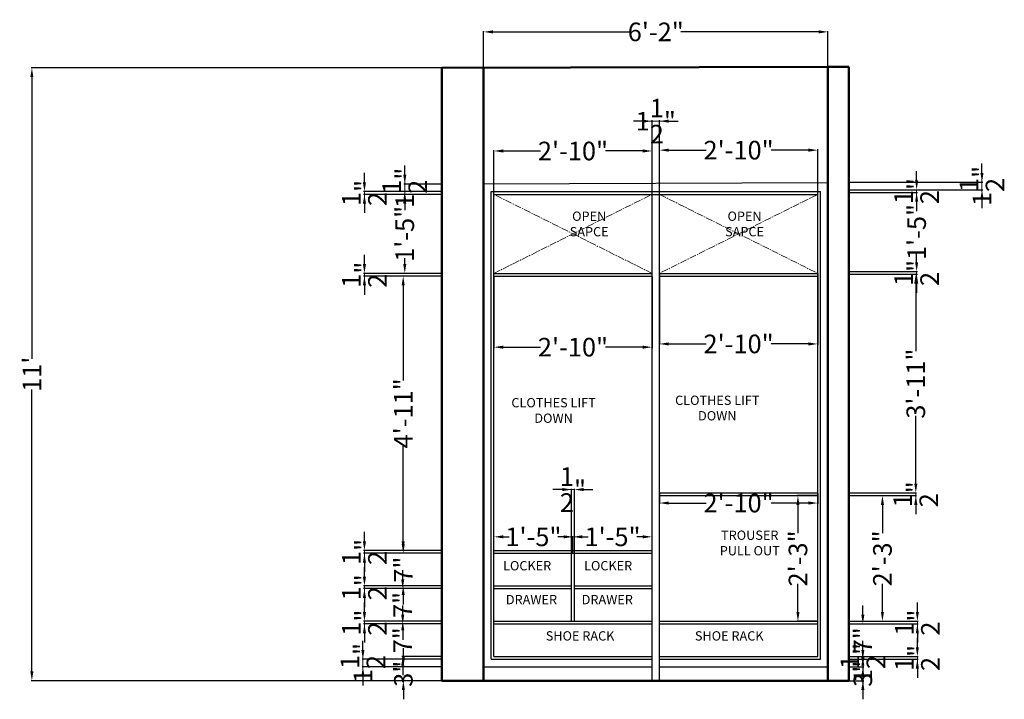
# Model space of a CAD drawing. Units: inches. Extents: x -26 to 186, y 15 to 278.
# Tile 1 of 2: x -26 to 186, y 15 to 161. Entities that reach past the tile are written whole.
import ezdxf

# ---------------------------------------------------------------- set-up
doc = ezdxf.new("R2010")
doc.units = ezdxf.units.IN
doc.header["$LTSCALE"] = 2
doc.header["$MEASUREMENT"] = 0
doc.linetypes.add('CENTER2', pattern=[1.125, 0.75, -0.125, 0.125, -0.125])
for name, color, linetype, lineweight in [('A-ANNO-DIMS', 2, 'Continuous', 18), ('A-ANNO-SYMB', 8, 'CENTER2', 13), ('A-ANNO-TEXT', 7, 'Continuous', 18), ('A-FURN', 3, 'Continuous', 25), ('A-WALL', 7, 'Continuous', 50)]:
    doc.layers.add(name, color=color, linetype=linetype, lineweight=lineweight)
doc.styles.get("Standard").update_dxf_attribs({"font": 'arial.ttf'})
doc.dimstyles.get("Standard").update_dxf_attribs({"dimtxt": 4, "dimasz": 2, "dimexe": 0.18, "dimexo": 0.0625, "dimgap": 0.09, "dimtad": 0, "dimdec": 1, "dimzin": 0, "dimdsep": 46, "dimlunit": 4, "dimtxsty": 'Standard', "dimcen": 0.09, "dimadec": 0, "dimazin": 0, "dimtfac": 1, "dimtdec": 1, "dimtix": 1, "dimtofl": 0, "dimtmove": 1, "dimatfit": 2, "dimfxl": 1, "dimtolj": 1, "dimtzin": 0, "dimarcsym": 0})

# ---------------------------------------------------------------- blocks, each defined once
blk = doc.blocks.new('*D6')
at = {"layer": 'A-ANNO-DIMS', "color": 0, "lineweight": -2, "transparency": 16777216}
for p, q in [((64.89, 150.53), (-23.34, 150.53)), ((-23.16, 148.53), (-23.16, 87.92)), ((-23.16, 20.73), (-23.16, 81.33)), ((64.89, 18.73), (-23.34, 18.73))]:
    blk.add_line(p, q, dxfattribs=at)
at = {"layer": 'A-ANNO-DIMS', "color": 0, "transparency": 16777216}
for points in [[(-23.49, 148.53), (-22.83, 148.53), (-23.16, 150.53)], [(-23.49, 20.73), (-22.83, 20.73), (-23.16, 18.73)]]:
    blk.add_solid(points, dxfattribs=at)
at = {"layer": 'Defpoints', "color": 0, "transparency": 16777216}
for p in [(64.95, 150.53), (-23.16, 18.73), (64.95, 18.73)]:
    blk.add_point(p, dxfattribs=at)
at = {"layer": 'A-ANNO-DIMS', "color": 0, "transparency": 16777216, "insert": (-23.16, 84.63), "char_height": 4, "attachment_point": 5, "rotation": 90}
blk.add_mtext("\\A1;11'", dxfattribs=at)
blk = doc.blocks.new('*D7')
at = {"layer": 'A-ANNO-DIMS', "color": 0, "lineweight": -2, "transparency": 16777216}
for p, q in [((155.46, 23.73), (155.46, 25.73)), ((152.51, 21.73), (155.64, 21.73)), ((152.51, 18.73), (155.64, 18.73)), ((155.46, 16.73), (155.46, 14.73))]:
    blk.add_line(p, q, dxfattribs=at)
at = {"layer": 'A-ANNO-DIMS', "color": 0, "transparency": 16777216}
for points in [[(155.13, 23.73), (155.79, 23.73), (155.46, 21.73)], [(155.13, 16.73), (155.79, 16.73), (155.46, 18.73)]]:
    blk.add_solid(points, dxfattribs=at)
at = {"layer": 'Defpoints', "color": 0, "transparency": 16777216}
for p in [(152.45, 21.73), (152.45, 18.73), (155.46, 18.73)]:
    blk.add_point(p, dxfattribs=at)
at = {"layer": 'A-ANNO-DIMS', "color": 0, "transparency": 16777216, "insert": (155.46, 20.23), "char_height": 4, "attachment_point": 5, "rotation": 90}
blk.add_mtext('\\A1;3"', dxfattribs=at)
blk = doc.blocks.new('*D8')
at = {"layer": 'A-ANNO-DIMS', "color": 0, "lineweight": -2, "transparency": 16777216}
for p, q in [((155.46, 25.33), (155.46, 27.33)), ((152.51, 23.33), (155.64, 23.33)), ((152.51, 21.73), (155.64, 21.73)), ((155.46, 19.73), (155.46, 17.73))]:
    blk.add_line(p, q, dxfattribs=at)
at = {"layer": 'A-ANNO-DIMS', "color": 0, "transparency": 16777216}
for points in [[(155.13, 25.33), (155.79, 25.33), (155.46, 23.33)], [(155.13, 19.73), (155.79, 19.73), (155.46, 21.73)]]:
    blk.add_solid(points, dxfattribs=at)
at = {"layer": 'Defpoints', "color": 0, "transparency": 16777216}
for p in [(152.45, 23.33), (155.46, 23.33), (152.45, 21.73)]:
    blk.add_point(p, dxfattribs=at)
at = {"layer": 'A-ANNO-DIMS', "color": 0, "transparency": 16777216, "insert": (155.46, 22.53), "char_height": 4, "attachment_point": 5, "rotation": 90}
blk.add_mtext('\\A1;1{\\H1x;\\S1/2;}"', dxfattribs=at)
blk = doc.blocks.new('*D9')
at = {"layer": 'A-ANNO-DIMS', "color": 0, "lineweight": -2, "transparency": 16777216}
for p, q in [((167.18, 25.93), (167.18, 27.93)), ((152.51, 23.93), (167.36, 23.93)), ((152.51, 23.33), (167.36, 23.33)), ((167.18, 21.33), (167.18, 19.33))]:
    blk.add_line(p, q, dxfattribs=at)
at = {"layer": 'A-ANNO-DIMS', "color": 0, "transparency": 16777216}
for points in [[(166.84, 25.93), (167.51, 25.93), (167.18, 23.93)], [(166.84, 21.33), (167.51, 21.33), (167.18, 23.33)]]:
    blk.add_solid(points, dxfattribs=at)
at = {"layer": 'Defpoints', "color": 0, "transparency": 16777216}
for p in [(152.45, 23.93), (152.45, 23.33), (167.18, 23.93)]:
    blk.add_point(p, dxfattribs=at)
at = {"layer": 'A-ANNO-DIMS', "color": 0, "transparency": 16777216, "insert": (167.18, 23.63), "char_height": 4, "attachment_point": 5, "rotation": 90}
blk.add_mtext('\\A1;{\\H1x;\\S1/2;}"', dxfattribs=at)
blk = doc.blocks.new('*D10')
at = {"layer": 'A-ANNO-DIMS', "color": 0, "lineweight": -2, "transparency": 16777216}
for p, q in [((155.46, 32.93), (155.46, 34.93)), ((152.51, 30.93), (155.64, 30.93)), ((152.51, 23.93), (155.64, 23.93)), ((155.46, 21.93), (155.46, 19.93))]:
    blk.add_line(p, q, dxfattribs=at)
at = {"layer": 'A-ANNO-DIMS', "color": 0, "transparency": 16777216}
for points in [[(155.13, 32.93), (155.79, 32.93), (155.46, 30.93)], [(155.13, 21.93), (155.79, 21.93), (155.46, 23.93)]]:
    blk.add_solid(points, dxfattribs=at)
at = {"layer": 'Defpoints', "color": 0, "transparency": 16777216}
for p in [(152.45, 30.93), (155.46, 30.93), (152.45, 23.93)]:
    blk.add_point(p, dxfattribs=at)
at = {"layer": 'A-ANNO-DIMS', "color": 0, "transparency": 16777216, "insert": (155.46, 27.43), "char_height": 4, "attachment_point": 5, "rotation": 90}
blk.add_mtext('\\A1;7"', dxfattribs=at)
blk = doc.blocks.new('*D11')
at = {"layer": 'A-ANNO-DIMS', "color": 0, "lineweight": -2, "transparency": 16777216}
for p, q in [((167.18, 33.53), (167.18, 35.53)), ((152.51, 31.53), (167.36, 31.53)), ((152.51, 30.93), (167.36, 30.93)), ((167.18, 28.93), (167.18, 26.93))]:
    blk.add_line(p, q, dxfattribs=at)
at = {"layer": 'A-ANNO-DIMS', "color": 0, "transparency": 16777216}
for points in [[(166.84, 33.53), (167.51, 33.53), (167.18, 31.53)], [(166.84, 28.93), (167.51, 28.93), (167.18, 30.93)]]:
    blk.add_solid(points, dxfattribs=at)
at = {"layer": 'Defpoints', "color": 0, "transparency": 16777216}
for p in [(152.45, 31.53), (152.45, 30.93), (167.18, 31.53)]:
    blk.add_point(p, dxfattribs=at)
at = {"layer": 'A-ANNO-DIMS', "color": 0, "transparency": 16777216, "insert": (167.18, 31.23), "char_height": 4, "attachment_point": 5, "rotation": 90}
blk.add_mtext('\\A1;{\\H1x;\\S1/2;}"', dxfattribs=at)
blk = doc.blocks.new('*D12')
at = {"layer": 'A-ANNO-DIMS', "color": 0, "lineweight": -2, "transparency": 16777216}
for p, q in [((152.51, 58.53), (159.85, 58.53)), ((159.67, 56.53), (159.67, 50.47)), ((159.67, 33.53), (159.67, 39.59)), ((152.51, 31.53), (159.85, 31.53))]:
    blk.add_line(p, q, dxfattribs=at)
at = {"layer": 'A-ANNO-DIMS', "color": 0, "transparency": 16777216}
for points in [[(159.34, 56.53), (160, 56.53), (159.67, 58.53)], [(159.34, 33.53), (160, 33.53), (159.67, 31.53)]]:
    blk.add_solid(points, dxfattribs=at)
at = {"layer": 'Defpoints', "color": 0, "transparency": 16777216}
for p in [(152.45, 58.53), (159.67, 58.53), (152.45, 31.53)]:
    blk.add_point(p, dxfattribs=at)
at = {"layer": 'A-ANNO-DIMS', "color": 0, "transparency": 16777216, "insert": (159.67, 45.03), "char_height": 4, "attachment_point": 5, "rotation": 90}
blk.add_mtext('\\A1;2\'-3"', dxfattribs=at)
blk = doc.blocks.new('*D13')
at = {"layer": 'A-ANNO-DIMS', "color": 0, "lineweight": -2, "transparency": 16777216}
for p, q in [((166.84, 61.13), (166.84, 63.13)), ((152.51, 59.13), (167.02, 59.13)), ((152.51, 58.53), (167.02, 58.53)), ((166.84, 56.53), (166.84, 54.53))]:
    blk.add_line(p, q, dxfattribs=at)
at = {"layer": 'A-ANNO-DIMS', "color": 0, "transparency": 16777216}
for points in [[(166.51, 61.13), (167.18, 61.13), (166.84, 59.13)], [(166.51, 56.53), (167.18, 56.53), (166.84, 58.53)]]:
    blk.add_solid(points, dxfattribs=at)
at = {"layer": 'Defpoints', "color": 0, "transparency": 16777216}
for p in [(152.45, 59.13), (152.45, 58.53), (166.84, 59.13)]:
    blk.add_point(p, dxfattribs=at)
at = {"layer": 'A-ANNO-DIMS', "color": 0, "transparency": 16777216, "insert": (166.84, 58.83), "char_height": 4, "attachment_point": 5, "rotation": 90}
blk.add_mtext('\\A1;{\\H1x;\\S1/2;}"', dxfattribs=at)
blk = doc.blocks.new('*D14')
at = {"layer": 'A-ANNO-DIMS', "color": 0, "lineweight": -2, "transparency": 16777216}
for p, q in [((152.51, 106.13), (167.02, 106.13)), ((166.84, 104.13), (166.84, 89.59)), ((166.84, 61.13), (166.84, 75.67)), ((152.51, 59.13), (167.02, 59.13))]:
    blk.add_line(p, q, dxfattribs=at)
at = {"layer": 'A-ANNO-DIMS', "color": 0, "transparency": 16777216}
for points in [[(166.51, 104.13), (167.18, 104.13), (166.84, 106.13)], [(166.51, 61.13), (167.18, 61.13), (166.84, 59.13)]]:
    blk.add_solid(points, dxfattribs=at)
at = {"layer": 'Defpoints', "color": 0, "transparency": 16777216}
for p in [(152.45, 106.13), (166.84, 106.13), (152.45, 59.13)]:
    blk.add_point(p, dxfattribs=at)
at = {"layer": 'A-ANNO-DIMS', "color": 0, "transparency": 16777216, "insert": (166.84, 82.63), "char_height": 4, "attachment_point": 5, "rotation": 90}
blk.add_mtext('\\A1;3\'-11"', dxfattribs=at)
blk = doc.blocks.new('*D15')
at = {"layer": 'A-ANNO-DIMS', "color": 0, "lineweight": -2, "transparency": 16777216}
for p, q in [((167.02, 108.73), (167.02, 110.73)), ((152.51, 106.73), (167.2, 106.73)), ((152.51, 106.13), (167.2, 106.13)), ((167.02, 104.13), (167.02, 102.13))]:
    blk.add_line(p, q, dxfattribs=at)
at = {"layer": 'A-ANNO-DIMS', "color": 0, "transparency": 16777216}
for points in [[(166.69, 108.73), (167.36, 108.73), (167.02, 106.73)], [(166.69, 104.13), (167.36, 104.13), (167.02, 106.13)]]:
    blk.add_solid(points, dxfattribs=at)
at = {"layer": 'Defpoints', "color": 0, "transparency": 16777216}
for p in [(152.45, 106.73), (152.45, 106.13), (167.02, 106.73)]:
    blk.add_point(p, dxfattribs=at)
at = {"layer": 'A-ANNO-DIMS', "color": 0, "transparency": 16777216, "insert": (167.02, 106.43), "char_height": 4, "attachment_point": 5, "rotation": 90}
blk.add_mtext('\\A1;{\\H1x;\\S1/2;}"', dxfattribs=at)
blk = doc.blocks.new('*D16')
at = {"layer": 'A-ANNO-DIMS', "color": 0, "lineweight": -2, "transparency": 16777216}
for p, q in [((152.51, 123.73), (167.2, 123.73)), ((167.02, 121.73), (167.02, 120.45)), ((167.02, 108.73), (167.02, 110.01)), ((152.51, 106.73), (167.2, 106.73))]:
    blk.add_line(p, q, dxfattribs=at)
at = {"layer": 'A-ANNO-DIMS', "color": 0, "transparency": 16777216}
for points in [[(166.69, 121.73), (167.36, 121.73), (167.02, 123.73)], [(166.69, 108.73), (167.36, 108.73), (167.02, 106.73)]]:
    blk.add_solid(points, dxfattribs=at)
at = {"layer": 'Defpoints', "color": 0, "transparency": 16777216}
for p in [(152.45, 123.73), (167.02, 123.73), (152.45, 106.73)]:
    blk.add_point(p, dxfattribs=at)
at = {"layer": 'A-ANNO-DIMS', "color": 0, "transparency": 16777216, "insert": (167.02, 115.23), "char_height": 4, "attachment_point": 5, "rotation": 90}
blk.add_mtext('\\A1;1\'-5"', dxfattribs=at)
blk = doc.blocks.new('*D17')
at = {"layer": 'A-ANNO-DIMS', "color": 0, "lineweight": -2, "transparency": 16777216}
for p, q in [((167.02, 126.33), (167.02, 128.33)), ((152.51, 124.33), (167.2, 124.33)), ((152.51, 123.73), (167.2, 123.73)), ((167.02, 121.73), (167.02, 119.73))]:
    blk.add_line(p, q, dxfattribs=at)
at = {"layer": 'A-ANNO-DIMS', "color": 0, "transparency": 16777216}
for points in [[(166.69, 126.33), (167.36, 126.33), (167.02, 124.33)], [(166.69, 121.73), (167.36, 121.73), (167.02, 123.73)]]:
    blk.add_solid(points, dxfattribs=at)
at = {"layer": 'Defpoints', "color": 0, "transparency": 16777216}
for p in [(152.45, 124.33), (152.45, 123.73), (167.02, 124.33)]:
    blk.add_point(p, dxfattribs=at)
at = {"layer": 'A-ANNO-DIMS', "color": 0, "transparency": 16777216, "insert": (167.02, 124.03), "char_height": 4, "attachment_point": 5, "rotation": 90}
blk.add_mtext('\\A1;{\\H1x;\\S1/2;}"', dxfattribs=at)
blk = doc.blocks.new('*D18')
at = {"layer": 'A-ANNO-DIMS', "color": 0, "lineweight": -2, "transparency": 16777216}
for p, q in [((181.07, 127.93), (181.07, 129.93)), ((152.51, 125.93), (181.25, 125.93)), ((152.51, 124.33), (181.25, 124.33)), ((181.07, 122.33), (181.07, 120.33))]:
    blk.add_line(p, q, dxfattribs=at)
at = {"layer": 'A-ANNO-DIMS', "color": 0, "transparency": 16777216}
for points in [[(180.73, 127.93), (181.4, 127.93), (181.07, 125.93)], [(180.73, 122.33), (181.4, 122.33), (181.07, 124.33)]]:
    blk.add_solid(points, dxfattribs=at)
at = {"layer": 'Defpoints', "color": 0, "transparency": 16777216}
for p in [(152.45, 125.93), (181.07, 125.93), (152.45, 124.33)]:
    blk.add_point(p, dxfattribs=at)
at = {"layer": 'A-ANNO-DIMS', "color": 0, "transparency": 16777216, "insert": (181.07, 125.13), "char_height": 4, "attachment_point": 5, "rotation": 90}
blk.add_mtext('\\A1;1{\\H1x;\\S1/2;}"', dxfattribs=at)
blk = doc.blocks.new('*D19')
at = {"layer": 'A-ANNO-DIMS', "color": 0, "lineweight": -2, "transparency": 16777216}
for p, q in [((56.69, 23.73), (56.69, 25.73)), ((64.89, 21.73), (56.51, 21.73)), ((64.89, 18.73), (56.51, 18.73)), ((56.69, 16.73), (56.69, 14.73))]:
    blk.add_line(p, q, dxfattribs=at)
at = {"layer": 'A-ANNO-DIMS', "color": 0, "transparency": 16777216}
for points in [[(56.36, 23.73), (57.02, 23.73), (56.69, 21.73)], [(56.36, 16.73), (57.02, 16.73), (56.69, 18.73)]]:
    blk.add_solid(points, dxfattribs=at)
at = {"layer": 'Defpoints', "color": 0, "transparency": 16777216}
for p in [(56.69, 21.73), (64.95, 21.73), (64.95, 18.73)]:
    blk.add_point(p, dxfattribs=at)
at = {"layer": 'A-ANNO-DIMS', "color": 0, "transparency": 16777216, "insert": (56.69, 20.23), "char_height": 4, "attachment_point": 5, "rotation": 90}
blk.add_mtext('\\A1;3"', dxfattribs=at)
blk = doc.blocks.new('*D20')
at = {"layer": 'A-ANNO-DIMS', "color": 0, "lineweight": -2, "transparency": 16777216}
for p, q in [((47.99, 25.33), (47.99, 27.33)), ((64.89, 23.33), (47.81, 23.33)), ((64.89, 21.73), (47.81, 21.73)), ((47.99, 19.73), (47.99, 17.73))]:
    blk.add_line(p, q, dxfattribs=at)
at = {"layer": 'A-ANNO-DIMS', "color": 0, "transparency": 16777216}
for points in [[(47.66, 25.33), (48.32, 25.33), (47.99, 23.33)], [(47.66, 19.73), (48.32, 19.73), (47.99, 21.73)]]:
    blk.add_solid(points, dxfattribs=at)
at = {"layer": 'Defpoints', "color": 0, "transparency": 16777216}
for p in [(47.99, 23.33), (64.95, 23.33), (64.95, 21.73)]:
    blk.add_point(p, dxfattribs=at)
at = {"layer": 'A-ANNO-DIMS', "color": 0, "transparency": 16777216, "insert": (47.99, 22.53), "char_height": 4, "attachment_point": 5, "rotation": 90}
blk.add_mtext('\\A1;1{\\H1x;\\S1/2;}"', dxfattribs=at)
blk = doc.blocks.new('*D21')
at = {"layer": 'A-ANNO-DIMS', "color": 0, "lineweight": -2, "transparency": 16777216}
for p, q in [((56.56, 32.93), (56.56, 34.93)), ((64.89, 30.93), (56.38, 30.93)), ((64.89, 23.93), (56.38, 23.93)), ((56.56, 21.93), (56.56, 19.93))]:
    blk.add_line(p, q, dxfattribs=at)
at = {"layer": 'A-ANNO-DIMS', "color": 0, "transparency": 16777216}
for points in [[(56.22, 32.93), (56.89, 32.93), (56.56, 30.93)], [(56.22, 21.93), (56.89, 21.93), (56.56, 23.93)]]:
    blk.add_solid(points, dxfattribs=at)
at = {"layer": 'Defpoints', "color": 0, "transparency": 16777216}
for p in [(56.56, 30.93), (64.95, 30.93), (64.95, 23.93)]:
    blk.add_point(p, dxfattribs=at)
at = {"layer": 'A-ANNO-DIMS', "color": 0, "transparency": 16777216, "insert": (56.56, 27.43), "char_height": 4, "attachment_point": 5, "rotation": 90}
blk.add_mtext('\\A1;7"', dxfattribs=at)
blk = doc.blocks.new('*D22')
at = {"layer": 'A-ANNO-DIMS', "color": 0, "lineweight": -2, "transparency": 16777216}
for p, q in [((48.32, 33.53), (48.32, 35.53)), ((64.89, 31.53), (48.14, 31.53)), ((64.89, 30.93), (48.14, 30.93)), ((48.32, 28.93), (48.32, 26.93))]:
    blk.add_line(p, q, dxfattribs=at)
at = {"layer": 'A-ANNO-DIMS', "color": 0, "transparency": 16777216}
for points in [[(47.99, 33.53), (48.66, 33.53), (48.32, 31.53)], [(47.99, 28.93), (48.66, 28.93), (48.32, 30.93)]]:
    blk.add_solid(points, dxfattribs=at)
at = {"layer": 'Defpoints', "color": 0, "transparency": 16777216}
for p in [(48.32, 31.53), (64.95, 31.53), (64.95, 30.93)]:
    blk.add_point(p, dxfattribs=at)
at = {"layer": 'A-ANNO-DIMS', "color": 0, "transparency": 16777216, "insert": (48.32, 31.23), "char_height": 4, "attachment_point": 5, "rotation": 90}
blk.add_mtext('\\A1;{\\H1x;\\S1/2;}"', dxfattribs=at)
blk = doc.blocks.new('*D23')
at = {"layer": 'A-ANNO-DIMS', "color": 0, "lineweight": -2, "transparency": 16777216}
for p, q in [((56.56, 40.53), (56.56, 42.53)), ((64.89, 38.53), (56.38, 38.53)), ((64.89, 31.53), (56.38, 31.53)), ((56.56, 29.53), (56.56, 27.53))]:
    blk.add_line(p, q, dxfattribs=at)
at = {"layer": 'A-ANNO-DIMS', "color": 0, "transparency": 16777216}
for points in [[(56.22, 40.53), (56.89, 40.53), (56.56, 38.53)], [(56.22, 29.53), (56.89, 29.53), (56.56, 31.53)]]:
    blk.add_solid(points, dxfattribs=at)
at = {"layer": 'Defpoints', "color": 0, "transparency": 16777216}
for p in [(56.56, 38.53), (64.95, 38.53), (64.95, 31.53)]:
    blk.add_point(p, dxfattribs=at)
at = {"layer": 'A-ANNO-DIMS', "color": 0, "transparency": 16777216, "insert": (56.56, 35.03), "char_height": 4, "attachment_point": 5, "rotation": 90}
blk.add_mtext('\\A1;7"', dxfattribs=at)
blk = doc.blocks.new('*D24')
at = {"layer": 'A-ANNO-DIMS', "color": 0, "lineweight": -2, "transparency": 16777216}
for p, q in [((48.32, 41.13), (48.32, 43.13)), ((64.89, 39.13), (48.14, 39.13)), ((64.89, 38.53), (48.14, 38.53)), ((48.32, 36.53), (48.32, 34.53))]:
    blk.add_line(p, q, dxfattribs=at)
at = {"layer": 'A-ANNO-DIMS', "color": 0, "transparency": 16777216}
for points in [[(47.99, 41.13), (48.66, 41.13), (48.32, 39.13)], [(47.99, 36.53), (48.66, 36.53), (48.32, 38.53)]]:
    blk.add_solid(points, dxfattribs=at)
at = {"layer": 'Defpoints', "color": 0, "transparency": 16777216}
for p in [(48.32, 39.13), (64.95, 39.13), (64.95, 38.53)]:
    blk.add_point(p, dxfattribs=at)
at = {"layer": 'A-ANNO-DIMS', "color": 0, "transparency": 16777216, "insert": (48.32, 38.83), "char_height": 4, "attachment_point": 5, "rotation": 90}
blk.add_mtext('\\A1;{\\H1x;\\S1/2;}"', dxfattribs=at)
blk = doc.blocks.new('*D25')
at = {"layer": 'A-ANNO-DIMS', "color": 0, "lineweight": -2, "transparency": 16777216}
for p, q in [((56.66, 48.13), (56.66, 50.13)), ((64.89, 46.13), (56.48, 46.13)), ((64.89, 39.13), (56.48, 39.13)), ((56.66, 37.13), (56.66, 35.13))]:
    blk.add_line(p, q, dxfattribs=at)
at = {"layer": 'A-ANNO-DIMS', "color": 0, "transparency": 16777216}
for points in [[(56.32, 48.13), (56.99, 48.13), (56.66, 46.13)], [(56.32, 37.13), (56.99, 37.13), (56.66, 39.13)]]:
    blk.add_solid(points, dxfattribs=at)
at = {"layer": 'Defpoints', "color": 0, "transparency": 16777216}
for p in [(56.66, 46.13), (64.95, 46.13), (64.95, 39.13)]:
    blk.add_point(p, dxfattribs=at)
at = {"layer": 'A-ANNO-DIMS', "color": 0, "transparency": 16777216, "insert": (56.66, 42.63), "char_height": 4, "attachment_point": 5, "rotation": 90}
blk.add_mtext('\\A1;7"', dxfattribs=at)
blk = doc.blocks.new('*D26')
at = {"layer": 'A-ANNO-DIMS', "color": 0, "lineweight": -2, "transparency": 16777216}
for p, q in [((48.32, 48.73), (48.32, 50.73)), ((64.89, 46.73), (48.14, 46.73)), ((64.89, 46.13), (48.14, 46.13)), ((48.32, 44.13), (48.32, 42.13))]:
    blk.add_line(p, q, dxfattribs=at)
at = {"layer": 'A-ANNO-DIMS', "color": 0, "transparency": 16777216}
for points in [[(47.99, 48.73), (48.66, 48.73), (48.32, 46.73)], [(47.99, 44.13), (48.66, 44.13), (48.32, 46.13)]]:
    blk.add_solid(points, dxfattribs=at)
at = {"layer": 'Defpoints', "color": 0, "transparency": 16777216}
for p in [(48.32, 46.73), (64.95, 46.73), (64.95, 46.13)]:
    blk.add_point(p, dxfattribs=at)
at = {"layer": 'A-ANNO-DIMS', "color": 0, "transparency": 16777216, "insert": (48.32, 46.43), "char_height": 4, "attachment_point": 5, "rotation": 90}
blk.add_mtext('\\A1;{\\H1x;\\S1/2;}"', dxfattribs=at)
blk = doc.blocks.new('*D27')
at = {"layer": 'A-ANNO-DIMS', "color": 0, "lineweight": -2, "transparency": 16777216}
for p, q in [((48.32, 108.33), (48.32, 110.33)), ((64.89, 106.33), (48.14, 106.33)), ((64.89, 105.73), (48.14, 105.73)), ((48.32, 103.73), (48.32, 101.73))]:
    blk.add_line(p, q, dxfattribs=at)
at = {"layer": 'A-ANNO-DIMS', "color": 0, "transparency": 16777216}
for points in [[(47.99, 108.33), (48.66, 108.33), (48.32, 106.33)], [(47.99, 103.73), (48.66, 103.73), (48.32, 105.73)]]:
    blk.add_solid(points, dxfattribs=at)
at = {"layer": 'Defpoints', "color": 0, "transparency": 16777216}
for p in [(48.32, 106.33), (64.95, 106.33), (64.95, 105.73)]:
    blk.add_point(p, dxfattribs=at)
at = {"layer": 'A-ANNO-DIMS', "color": 0, "transparency": 16777216, "insert": (48.32, 106.03), "char_height": 4, "attachment_point": 5, "rotation": 90}
blk.add_mtext('\\A1;{\\H1x;\\S1/2;}"', dxfattribs=at)
blk = doc.blocks.new('*D28')
at = {"layer": 'A-ANNO-DIMS', "color": 0, "lineweight": -2, "transparency": 16777216}
for p, q in [((64.89, 105.73), (56.48, 105.73)), ((56.66, 103.73), (56.66, 83.27)), ((56.66, 48.73), (56.66, 69.19)), ((64.89, 46.73), (56.48, 46.73))]:
    blk.add_line(p, q, dxfattribs=at)
at = {"layer": 'A-ANNO-DIMS', "color": 0, "transparency": 16777216}
for points in [[(56.32, 103.73), (56.99, 103.73), (56.66, 105.73)], [(56.32, 48.73), (56.99, 48.73), (56.66, 46.73)]]:
    blk.add_solid(points, dxfattribs=at)
at = {"layer": 'Defpoints', "color": 0, "transparency": 16777216}
for p in [(56.66, 105.73), (64.95, 105.73), (64.95, 46.73)]:
    blk.add_point(p, dxfattribs=at)
at = {"layer": 'A-ANNO-DIMS', "color": 0, "transparency": 16777216, "insert": (56.66, 76.23), "char_height": 4, "attachment_point": 5, "rotation": 90}
blk.add_mtext('\\A1;4\'-11"', dxfattribs=at)
blk = doc.blocks.new('*D29')
at = {"layer": 'A-ANNO-DIMS', "color": 0, "lineweight": -2, "transparency": 16777216}
for p, q in [((64.89, 123.33), (56.81, 123.33)), ((56.99, 121.33), (56.99, 120.05)), ((56.99, 108.33), (56.99, 109.61)), ((64.89, 106.33), (56.81, 106.33))]:
    blk.add_line(p, q, dxfattribs=at)
at = {"layer": 'A-ANNO-DIMS', "color": 0, "transparency": 16777216}
for points in [[(56.66, 121.33), (57.32, 121.33), (56.99, 123.33)], [(56.66, 108.33), (57.32, 108.33), (56.99, 106.33)]]:
    blk.add_solid(points, dxfattribs=at)
at = {"layer": 'Defpoints', "color": 0, "transparency": 16777216}
for p in [(56.99, 123.33), (64.95, 123.33), (64.95, 106.33)]:
    blk.add_point(p, dxfattribs=at)
at = {"layer": 'A-ANNO-DIMS', "color": 0, "transparency": 16777216, "insert": (56.99, 114.83), "char_height": 4, "attachment_point": 5, "rotation": 90}
blk.add_mtext('\\A1;1\'-5"', dxfattribs=at)
blk = doc.blocks.new('*D30')
at = {"layer": 'A-ANNO-DIMS', "color": 0, "lineweight": -2, "transparency": 16777216}
for p, q in [((48.32, 125.93), (48.32, 127.93)), ((64.89, 123.93), (48.14, 123.93)), ((64.89, 123.33), (48.14, 123.33)), ((48.32, 121.33), (48.32, 119.33))]:
    blk.add_line(p, q, dxfattribs=at)
at = {"layer": 'A-ANNO-DIMS', "color": 0, "transparency": 16777216}
for points in [[(47.99, 125.93), (48.66, 125.93), (48.32, 123.93)], [(47.99, 121.33), (48.66, 121.33), (48.32, 123.33)]]:
    blk.add_solid(points, dxfattribs=at)
at = {"layer": 'Defpoints', "color": 0, "transparency": 16777216}
for p in [(48.32, 123.93), (64.95, 123.93), (64.95, 123.33)]:
    blk.add_point(p, dxfattribs=at)
at = {"layer": 'A-ANNO-DIMS', "color": 0, "transparency": 16777216, "insert": (48.32, 123.63), "char_height": 4, "attachment_point": 5, "rotation": 90}
blk.add_mtext('\\A1;{\\H1x;\\S1/2;}"', dxfattribs=at)
blk = doc.blocks.new('*D31')
at = {"layer": 'A-ANNO-DIMS', "color": 0, "lineweight": -2, "transparency": 16777216}
for p, q in [((56.99, 127.53), (56.99, 129.53)), ((64.89, 125.53), (56.81, 125.53)), ((64.89, 123.93), (56.81, 123.93)), ((56.99, 121.93), (56.99, 119.93))]:
    blk.add_line(p, q, dxfattribs=at)
at = {"layer": 'A-ANNO-DIMS', "color": 0, "transparency": 16777216}
for points in [[(56.66, 127.53), (57.32, 127.53), (56.99, 125.53)], [(56.66, 121.93), (57.32, 121.93), (56.99, 123.93)]]:
    blk.add_solid(points, dxfattribs=at)
at = {"layer": 'Defpoints', "color": 0, "transparency": 16777216}
for p in [(56.99, 125.53), (64.95, 125.53), (64.95, 123.93)]:
    blk.add_point(p, dxfattribs=at)
at = {"layer": 'A-ANNO-DIMS', "color": 0, "transparency": 16777216, "insert": (56.99, 124.73), "char_height": 4, "attachment_point": 5, "rotation": 90}
blk.add_mtext('\\A1;1{\\H1x;\\S1/2;}"', dxfattribs=at)
blk = doc.blocks.new('*D32')
at = {"layer": 'A-ANNO-DIMS', "color": 0, "lineweight": -2, "transparency": 16777216}
for p, q in [((76.15, 46.19), (76.15, 49.85)), ((78.15, 49.67), (79.43, 49.67)), ((91.15, 49.67), (89.87, 49.67)), ((93.15, 46.19), (93.15, 49.85))]:
    blk.add_line(p, q, dxfattribs=at)
at = {"layer": 'A-ANNO-DIMS', "color": 0, "transparency": 16777216}
for points in [[(78.15, 50), (78.15, 49.34), (76.15, 49.67)], [(91.15, 50), (91.15, 49.34), (93.15, 49.67)]]:
    blk.add_solid(points, dxfattribs=at)
at = {"layer": 'Defpoints', "color": 0, "transparency": 16777216}
for p in [(93.15, 49.67), (76.15, 46.13), (93.15, 46.13)]:
    blk.add_point(p, dxfattribs=at)
at = {"layer": 'A-ANNO-DIMS', "color": 0, "transparency": 16777216, "insert": (84.65, 49.67), "char_height": 4, "attachment_point": 5}
blk.add_mtext('\\A1;1\'-5"', dxfattribs=at)
blk = doc.blocks.new('*D33')
at = {"layer": 'A-ANNO-DIMS', "color": 0, "lineweight": -2, "transparency": 16777216}
for p, q in [((93.15, 46.19), (93.15, 49.85)), ((95.15, 49.67), (96.43, 49.67)), ((108.15, 49.67), (106.87, 49.67)), ((110.15, 46.19), (110.15, 49.85))]:
    blk.add_line(p, q, dxfattribs=at)
at = {"layer": 'A-ANNO-DIMS', "color": 0, "transparency": 16777216}
for points in [[(95.15, 50), (95.15, 49.34), (93.15, 49.67)], [(108.15, 50), (108.15, 49.34), (110.15, 49.67)]]:
    blk.add_solid(points, dxfattribs=at)
at = {"layer": 'Defpoints', "color": 0, "transparency": 16777216}
for p in [(110.15, 49.67), (93.15, 46.13), (110.15, 46.13)]:
    blk.add_point(p, dxfattribs=at)
at = {"layer": 'A-ANNO-DIMS', "color": 0, "transparency": 16777216, "insert": (101.65, 49.67), "char_height": 4, "attachment_point": 5}
blk.add_mtext('\\A1;1\'-5"', dxfattribs=at)
blk = doc.blocks.new('*D34')
at = {"layer": 'A-ANNO-DIMS', "color": 0, "lineweight": -2, "transparency": 16777216}
for p, q in [((73.95, 150.79), (73.95, 158.45)), ((75.95, 158.27), (105.53, 158.27)), ((145.95, 158.27), (116.37, 158.27)), ((147.95, 150.79), (147.95, 158.45))]:
    blk.add_line(p, q, dxfattribs=at)
at = {"layer": 'A-ANNO-DIMS', "color": 0, "transparency": 16777216}
for points in [[(75.95, 158.6), (75.95, 157.93), (73.95, 158.27)], [(145.95, 158.6), (145.95, 157.93), (147.95, 158.27)]]:
    blk.add_solid(points, dxfattribs=at)
at = {"layer": 'Defpoints', "color": 0, "transparency": 16777216}
for p in [(147.95, 158.27), (73.95, 150.73), (147.95, 150.73)]:
    blk.add_point(p, dxfattribs=at)
at = {"layer": 'A-ANNO-DIMS', "color": 0, "transparency": 16777216, "insert": (110.95, 158.27), "char_height": 4, "attachment_point": 5}
blk.add_mtext('\\A1;6\'-2"', dxfattribs=at)
blk = doc.blocks.new('*D35')
at = {"layer": 'A-ANNO-DIMS', "color": 0, "lineweight": -2, "transparency": 16777216}
for p, q in [((76.15, 123.39), (76.15, 132.83)), ((78.15, 132.65), (86.15, 132.65)), ((108.15, 132.65), (100.14, 132.65)), ((110.15, 123.39), (110.15, 132.83))]:
    blk.add_line(p, q, dxfattribs=at)
at = {"layer": 'A-ANNO-DIMS', "color": 0, "transparency": 16777216}
for points in [[(78.15, 132.99), (78.15, 132.32), (76.15, 132.65)], [(108.15, 132.99), (108.15, 132.32), (110.15, 132.65)]]:
    blk.add_solid(points, dxfattribs=at)
at = {"layer": 'Defpoints', "color": 0, "transparency": 16777216}
for p in [(76.15, 132.65), (76.15, 123.33), (110.15, 123.33)]:
    blk.add_point(p, dxfattribs=at)
at = {"layer": 'A-ANNO-DIMS', "color": 0, "transparency": 16777216, "insert": (93.15, 132.65), "char_height": 4, "attachment_point": 5}
blk.add_mtext('\\A1;2\'-10"', dxfattribs=at)
blk = doc.blocks.new('*D36')
at = {"layer": 'A-ANNO-DIMS', "color": 0, "lineweight": -2, "transparency": 16777216}
for p, q in [((111.75, 123.39), (111.75, 133.01)), ((113.75, 132.83), (121.75, 132.83)), ((143.75, 132.83), (135.74, 132.83)), ((145.75, 123.39), (145.75, 133.01))]:
    blk.add_line(p, q, dxfattribs=at)
at = {"layer": 'A-ANNO-DIMS', "color": 0, "transparency": 16777216}
for points in [[(113.75, 133.17), (113.75, 132.5), (111.75, 132.83)], [(143.75, 133.17), (143.75, 132.5), (145.75, 132.83)]]:
    blk.add_solid(points, dxfattribs=at)
at = {"layer": 'Defpoints', "color": 0, "transparency": 16777216}
for p in [(145.75, 132.83), (111.75, 123.33), (145.75, 123.33)]:
    blk.add_point(p, dxfattribs=at)
at = {"layer": 'A-ANNO-DIMS', "color": 0, "transparency": 16777216, "insert": (128.75, 132.83), "char_height": 4, "attachment_point": 5}
blk.add_mtext('\\A1;2\'-10"', dxfattribs=at)
blk = doc.blocks.new('*D37')
at = {"layer": 'A-ANNO-DIMS', "color": 0, "lineweight": -2, "transparency": 16777216}
for p, q in [((76.15, 105.67), (76.15, 90.28)), ((110.15, 105.67), (110.15, 90.28)), ((78.15, 90.46), (86.15, 90.46)), ((108.15, 90.46), (100.14, 90.46))]:
    blk.add_line(p, q, dxfattribs=at)
at = {"layer": 'A-ANNO-DIMS', "color": 0, "transparency": 16777216}
for points in [[(78.15, 90.79), (78.15, 90.13), (76.15, 90.46)], [(108.15, 90.79), (108.15, 90.13), (110.15, 90.46)]]:
    blk.add_solid(points, dxfattribs=at)
at = {"layer": 'Defpoints', "color": 0, "transparency": 16777216}
for p in [(76.15, 105.73), (110.15, 105.73), (110.15, 90.46)]:
    blk.add_point(p, dxfattribs=at)
at = {"layer": 'A-ANNO-DIMS', "color": 0, "transparency": 16777216, "insert": (93.15, 90.46), "char_height": 4, "attachment_point": 5}
blk.add_mtext('\\A1;2\'-10"', dxfattribs=at)
blk = doc.blocks.new('*D38')
at = {"layer": 'A-ANNO-DIMS', "color": 0, "lineweight": -2, "transparency": 16777216}
for p, q in [((111.75, 106.27), (111.75, 90.98)), ((145.75, 106.27), (145.75, 90.98)), ((113.75, 91.16), (121.75, 91.16)), ((143.75, 91.16), (135.74, 91.16))]:
    blk.add_line(p, q, dxfattribs=at)
at = {"layer": 'A-ANNO-DIMS', "color": 0, "transparency": 16777216}
for points in [[(113.75, 91.49), (113.75, 90.82), (111.75, 91.16)], [(143.75, 91.49), (143.75, 90.82), (145.75, 91.16)]]:
    blk.add_solid(points, dxfattribs=at)
at = {"layer": 'Defpoints', "color": 0, "transparency": 16777216}
for p in [(111.75, 106.33), (145.75, 106.33), (145.75, 91.16)]:
    blk.add_point(p, dxfattribs=at)
at = {"layer": 'A-ANNO-DIMS', "color": 0, "transparency": 16777216, "insert": (128.75, 91.16), "char_height": 4, "attachment_point": 5}
blk.add_mtext('\\A1;2\'-10"', dxfattribs=at)
blk = doc.blocks.new('*D39')
at = {"layer": 'A-ANNO-DIMS', "color": 0, "lineweight": -2, "transparency": 16777216}
for p, q in [((90.85, 59.84), (88.85, 59.84)), ((92.85, 46.19), (92.85, 60.02)), ((93.45, 46.19), (93.45, 60.02)), ((95.45, 59.84), (97.45, 59.84))]:
    blk.add_line(p, q, dxfattribs=at)
at = {"layer": 'A-ANNO-DIMS', "color": 0, "transparency": 16777216}
for points in [[(90.85, 60.18), (90.85, 59.51), (92.85, 59.84)], [(95.45, 60.18), (95.45, 59.51), (93.45, 59.84)]]:
    blk.add_solid(points, dxfattribs=at)
at = {"layer": 'Defpoints', "color": 0, "transparency": 16777216}
for p in [(93.45, 59.84), (92.85, 46.13), (93.45, 46.13)]:
    blk.add_point(p, dxfattribs=at)
at = {"layer": 'A-ANNO-DIMS', "color": 0, "transparency": 16777216, "insert": (93.15, 59.84), "char_height": 4, "attachment_point": 5}
blk.add_mtext('\\A1;{\\H1x;\\S1/2;}"', dxfattribs=at)
blk = doc.blocks.new('*D40')
at = {"layer": 'A-ANNO-DIMS', "color": 0, "lineweight": -2, "transparency": 16777216}
for p, q in [((111.75, 59.07), (111.75, 56.76)), ((145.75, 59.07), (145.75, 56.76)), ((113.75, 56.94), (121.75, 56.94)), ((143.75, 56.94), (135.74, 56.94))]:
    blk.add_line(p, q, dxfattribs=at)
at = {"layer": 'A-ANNO-DIMS', "color": 0, "transparency": 16777216}
for points in [[(113.75, 57.28), (113.75, 56.61), (111.75, 56.94)], [(143.75, 57.28), (143.75, 56.61), (145.75, 56.94)]]:
    blk.add_solid(points, dxfattribs=at)
at = {"layer": 'Defpoints', "color": 0, "transparency": 16777216}
for p in [(111.75, 59.13), (145.75, 59.13), (145.75, 56.94)]:
    blk.add_point(p, dxfattribs=at)
at = {"layer": 'A-ANNO-DIMS', "color": 0, "transparency": 16777216, "insert": (128.75, 56.94), "char_height": 4, "attachment_point": 5}
blk.add_mtext('\\A1;2\'-10"', dxfattribs=at)
blk = doc.blocks.new('*D41')
at = {"layer": 'A-ANNO-DIMS', "color": 0, "lineweight": -2, "transparency": 16777216}
for p, q in [((145.69, 58.53), (141.33, 58.53)), ((141.51, 56.53), (141.51, 50.47)), ((141.51, 33.53), (141.51, 39.59)), ((145.69, 31.53), (141.33, 31.53))]:
    blk.add_line(p, q, dxfattribs=at)
at = {"layer": 'A-ANNO-DIMS', "color": 0, "transparency": 16777216}
for points in [[(141.17, 56.53), (141.84, 56.53), (141.51, 58.53)], [(141.17, 33.53), (141.84, 33.53), (141.51, 31.53)]]:
    blk.add_solid(points, dxfattribs=at)
at = {"layer": 'Defpoints', "color": 0, "transparency": 16777216}
for p in [(145.75, 58.53), (141.51, 31.53), (145.75, 31.53)]:
    blk.add_point(p, dxfattribs=at)
at = {"layer": 'A-ANNO-DIMS', "color": 0, "transparency": 16777216, "insert": (141.51, 45.03), "char_height": 4, "attachment_point": 5, "rotation": 90}
blk.add_mtext('\\A1;2\'-3"', dxfattribs=at)
blk = doc.blocks.new('*D42')
at = {"layer": 'A-ANNO-DIMS', "color": 0, "lineweight": -2, "transparency": 16777216}
for p, q in [((108.15, 139.07), (106.15, 139.07)), ((110.15, 123.39), (110.15, 139.25)), ((111.75, 123.39), (111.75, 139.25)), ((113.75, 139.07), (115.75, 139.07))]:
    blk.add_line(p, q, dxfattribs=at)
at = {"layer": 'A-ANNO-DIMS', "color": 0, "transparency": 16777216}
for points in [[(108.15, 139.4), (108.15, 138.74), (110.15, 139.07)], [(113.75, 139.4), (113.75, 138.74), (111.75, 139.07)]]:
    blk.add_solid(points, dxfattribs=at)
at = {"layer": 'Defpoints', "color": 0, "transparency": 16777216}
for p in [(111.75, 139.07), (110.15, 123.33), (111.75, 123.33)]:
    blk.add_point(p, dxfattribs=at)
at = {"layer": 'A-ANNO-DIMS', "color": 0, "transparency": 16777216, "insert": (110.95, 139.07), "char_height": 4, "attachment_point": 5}
blk.add_mtext('\\A1;1{\\H1x;\\S1/2;}"', dxfattribs=at)

msp = doc.modelspace()

# ---------------------------------------------------------------- linework, layer by layer
at = {"layer": 'A-ANNO-SYMB'}
for p, q in [((110.15, 106.33), (76.15, 123.33)), ((76.15, 106.33), (110.15, 123.33)), ((111.75, 123.33), (145.75, 106.33)), ((145.75, 123.33), (111.75, 106.33))]:
    msp.add_line(p, q, dxfattribs=at)
at = {"layer": 'A-FURN'}
for p, q in [((73.95, 125.57), (147.95, 125.91)), ((75.55, 123.93), (146.35, 123.93)), ((75.55, 23.33), (75.55, 123.93)), ((76.15, 123.33), (145.75, 123.33)), ((76.15, 46.73), (76.15, 123.33)), ((110.15, 18.73), (110.15, 123.33)), ((111.75, 18.73), (111.75, 123.33)), ((145.75, 23.93), (145.75, 123.33)), ((146.35, 23.33), (146.35, 123.93)), ((76.15, 106.33), (110.15, 106.33)), ((111.75, 106.33), (145.75, 106.33)), ((76.15, 105.73), (110.15, 105.73)), ((111.75, 105.73), (145.75, 105.73)), ((111.75, 59.13), (145.75, 59.13)), ((111.75, 58.53), (145.75, 58.53)), ((76.15, 46.73), (110.15, 46.73)), ((76.15, 46.13), (110.15, 46.13)), ((76.15, 23.93), (76.15, 46.13)), ((92.85, 31.53), (92.85, 46.13)), ((93.45, 31.53), (93.45, 46.13)), ((76.15, 39.13), (92.85, 39.13)), ((76.15, 38.53), (92.85, 38.53)), ((93.45, 39.13), (110.15, 39.13)), ((93.45, 38.53), (110.15, 38.53)), ((76.15, 31.53), (92.85, 31.53)), ((76.15, 30.93), (92.85, 30.93)), ((92.85, 31.53), (110.15, 31.53)), ((92.85, 30.93), (110.15, 30.93)), ((111.75, 31.53), (145.75, 31.53)), ((111.75, 30.93), (145.75, 30.93)), ((75.55, 23.33), (110.15, 23.33)), ((76.15, 23.93), (92.85, 23.93)), ((92.85, 23.93), (110.15, 23.93)), ((111.75, 23.93), (145.75, 23.93)), ((111.75, 23.33), (146.35, 23.33)), ((73.95, 21.73), (110.15, 21.73)), ((111.75, 21.73), (147.95, 21.73))]:
    msp.add_line(p, q, dxfattribs=at)
at = {"layer": 'A-WALL'}
for p, q in [((64.95, 150.53), (147.95, 150.73)), ((64.95, 149.53), (64.95, 150.53)), ((73.95, 18.73), (73.95, 150.73)), ((147.95, 18.73), (147.95, 150.73)), ((147.95, 150.73), (152.45, 150.73)), ((152.45, 125.93), (152.45, 150.73)), ((64.95, 125.53), (64.95, 149.53)), ((64.95, 123.93), (64.95, 125.53)), ((152.45, 124.33), (152.45, 125.93)), ((64.95, 123.33), (64.95, 123.93)), ((64.95, 106.33), (64.95, 123.33)), ((152.45, 123.73), (152.45, 124.33)), ((152.45, 106.73), (152.45, 123.73)), ((64.95, 105.73), (64.95, 106.33)), ((152.45, 106.13), (152.45, 106.73)), ((152.45, 59.13), (152.45, 106.13)), ((64.95, 46.73), (64.95, 105.73)), ((152.45, 58.53), (152.45, 59.13)), ((152.45, 31.53), (152.45, 58.53)), ((64.95, 46.13), (64.95, 46.73)), ((64.95, 39.13), (64.95, 46.13)), ((64.95, 38.53), (64.95, 39.13)), ((64.95, 31.53), (64.95, 38.53)), ((64.95, 30.93), (64.95, 31.53)), ((64.95, 23.93), (64.95, 30.93)), ((152.45, 30.93), (152.45, 31.53)), ((152.45, 23.93), (152.45, 30.93)), ((64.95, 23.33), (64.95, 23.93)), ((64.95, 21.73), (64.95, 23.33)), ((152.45, 23.33), (152.45, 23.93)), ((152.45, 21.73), (152.45, 23.33)), ((64.95, 18.73), (64.95, 21.73)), ((152.45, 18.73), (152.45, 21.73)), ((64.95, 18.73), (73.95, 18.73)), ((73.95, 18.73), (147.95, 18.73)), ((147.95, 18.73), (152.45, 18.73))]:
    msp.add_line(p, q, dxfattribs=at)

# ---------------------------------------------------------------- texts
at = {"layer": 'A-ANNO-TEXT', "char_height": 2, "attachment_point": 1}
for s, width, insert in [('\\pxqc;OPEN\\PSAPCE', 15.8682, (88.7, 119.63)), ('\\pxqc;OPEN\\PSAPCE', 15.8682, (122.1, 119.63)), ('\\pxqc;CLOTHES LIFT\\PDOWN', 43.4764, (67.24, 79.52)), ('\\pxqc;CLOTHES LIFT\\PDOWN', 43.4764, (102.43, 80.04)), ('\\pxqc;TROUSER\\PPULL OUT', 24.0823, (119.11, 51.02)), ('LOCKER', 13.2306, (78.12, 44.46)), ('LOCKER', 13.2306, (95.53, 44.46)), ('DRAWER', 12.0885, (78.72, 37.17)), ('DRAWER', 12.0885, (95.02, 37.17)), ('\\pxqc;SHOE RACK', 19.9328, (84.71, 29.37)), ('\\pxqc;SHOE RACK', 19.9328, (116.77, 29.37))]:
    msp.add_mtext_dynamic_manual_height_columns(s, width=width, gutter_width=10, heights=[0], dxfattribs=dict(at, insert=insert))

# ---------------------------------------------------------------- dimensions: what is measured, and where the dimension line sits
at = {"layer": 'A-ANNO-DIMS'}
for base, p1, p2, picture, middle in [((147.95, 158.27), (73.95, 150.73), (147.95, 150.73), '*D34', (110.95, 158.27)), ((111.75, 139.07), (110.15, 123.33), (111.75, 123.33), '*D42', (110.95, 139.07)), ((145.75, 132.83), (111.75, 123.33), (145.75, 123.33), '*D36', (128.75, 132.83)), ((76.15, 132.65), (110.15, 123.33), (76.15, 123.33), '*D35', (93.15, 132.65)), ((145.75, 91.16), (111.75, 106.33), (145.75, 106.33), '*D38', (128.75, 91.16)), ((110.15, 90.46), (76.15, 105.73), (110.15, 105.73), '*D37', (93.15, 90.46)), ((93.45, 59.84), (92.85, 46.13), (93.45, 46.13), '*D39', (93.15, 59.84)), ((145.75, 56.94), (111.75, 59.13), (145.75, 59.13), '*D40', (128.75, 56.94)), ((93.15, 49.67), (76.15, 46.13), (93.15, 46.13), '*D32', (84.65, 49.67)), ((110.15, 49.67), (93.15, 46.13), (110.15, 46.13), '*D33', (101.65, 49.67))]:
    dim = msp.add_linear_dim(base=base, p1=p1, p2=p2, dimstyle='Standard', override={"dimclrd": 0, "dimclre": 0, "dimclrt": 0}, dxfattribs=at)
    dim.commit()
    dim.dimension.update_dxf_attribs({"geometry": picture, "text_midpoint": middle})
for base, p1, p2, picture, middle in [((-23.16, 18.73), (64.95, 150.53), (64.95, 18.73), '*D6', (-23.16, 84.63)), ((56.99, 125.53), (64.95, 123.93), (64.95, 125.53), '*D31', (56.99, 124.73)), ((181.07, 125.93), (152.45, 124.33), (152.45, 125.93), '*D18', (181.07, 125.13)), ((167.02, 124.33), (152.45, 123.73), (152.45, 124.33), '*D17', (167.02, 124.03)), ((48.32, 123.93), (64.95, 123.33), (64.95, 123.93), '*D30', (48.32, 123.63)), ((56.99, 123.33), (64.95, 106.33), (64.95, 123.33), '*D29', (56.99, 114.83)), ((167.02, 123.73), (152.45, 106.73), (152.45, 123.73), '*D16', (167.02, 115.23)), ((48.32, 106.33), (64.95, 105.73), (64.95, 106.33), '*D27', (48.32, 106.03)), ((167.02, 106.73), (152.45, 106.13), (152.45, 106.73), '*D15', (167.02, 106.43)), ((166.84, 106.13), (152.45, 59.13), (152.45, 106.13), '*D14', (166.84, 82.63)), ((56.66, 105.73), (64.95, 46.73), (64.95, 105.73), '*D28', (56.66, 76.23)), ((166.84, 59.13), (152.45, 58.53), (152.45, 59.13), '*D13', (166.84, 58.83)), ((141.51, 31.53), (145.75, 58.53), (145.75, 31.53), '*D41', (141.51, 45.03)), ((159.67, 58.53), (152.45, 31.53), (152.45, 58.53), '*D12', (159.67, 45.03)), ((48.32, 46.73), (64.95, 46.13), (64.95, 46.73), '*D26', (48.32, 46.43)), ((56.66, 46.13), (64.95, 39.13), (64.95, 46.13), '*D25', (56.66, 42.63)), ((48.32, 39.13), (64.95, 38.53), (64.95, 39.13), '*D24', (48.32, 38.83)), ((56.56, 38.53), (64.95, 31.53), (64.95, 38.53), '*D23', (56.56, 35.03)), ((48.32, 31.53), (64.95, 30.93), (64.95, 31.53), '*D22', (48.32, 31.23)), ((167.18, 31.53), (152.45, 30.93), (152.45, 31.53), '*D11', (167.18, 31.23)), ((56.56, 30.93), (64.95, 23.93), (64.95, 30.93), '*D21', (56.56, 27.43)), ((155.46, 30.93), (152.45, 23.93), (152.45, 30.93), '*D10', (155.46, 27.43)), ((47.99, 23.33), (64.95, 21.73), (64.95, 23.33), '*D20', (47.99, 22.53)), ((155.46, 23.33), (152.45, 21.73), (152.45, 23.33), '*D8', (155.46, 22.53)), ((167.18, 23.93), (152.45, 23.33), (152.45, 23.93), '*D9', (167.18, 23.63)), ((56.69, 21.73), (64.95, 18.73), (64.95, 21.73), '*D19', (56.69, 20.23)), ((155.46, 18.73), (152.45, 21.73), (152.45, 18.73), '*D7', (155.46, 20.23))]:
    dim = msp.add_linear_dim(base=base, p1=p1, p2=p2, angle=90, dimstyle='Standard', override={"dimclrd": 0, "dimclre": 0, "dimclrt": 0}, dxfattribs=at)
    dim.commit()
    dim.dimension.update_dxf_attribs({"geometry": picture, "text_midpoint": middle})

doc.saveas('drawing.dxf')
